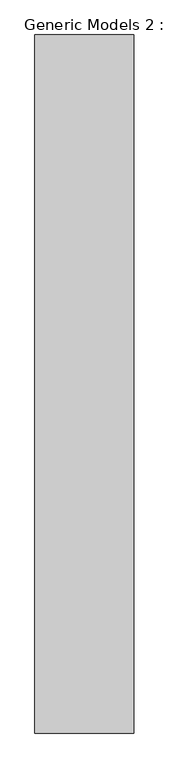
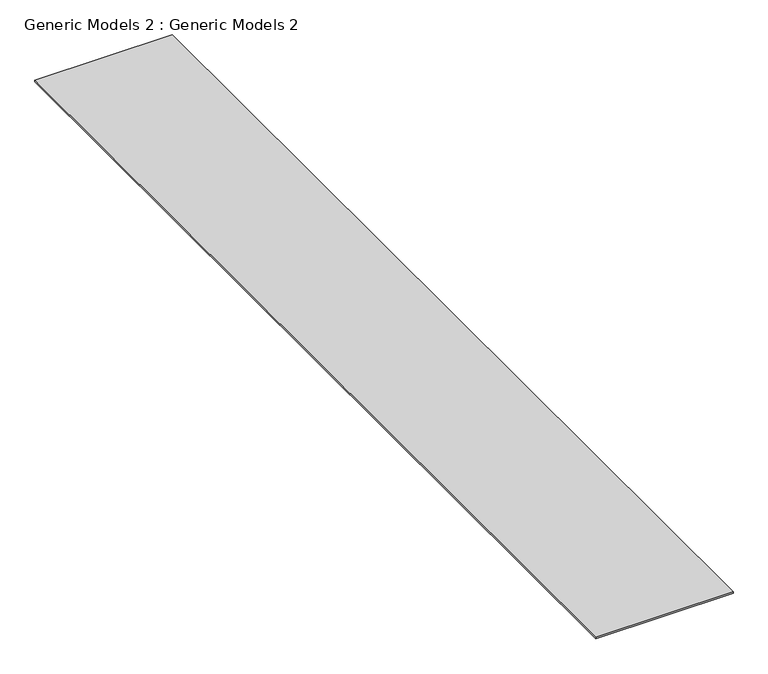
"""IFC4 building model written with IfcOpenShell, lengths in millimetres: proxy geometry, Generic Models 2 : Generic Models 2."""

from ifc_helpers import new_model, si_unit, frame, origin, place, context, project, spatial, polyline, outline, extrude, source, transform, mapped, element, save


def generic_models_2_generic_models_2_33b85b70(model_context):
    return source(origin(), model_context, "Body", "SweptSolid", [
        extrude(outline(polyline([(17947.2014317, 13822.3935985), (17947.2014317, -18476.1844555), (13375.2014317, -18476.1844555), (13375.2014317, 13822.3935985), (17947.2014317, 13822.3935985)])), frame((0.0, 0.0, -609.6), z_axis=(0.0, 0.0, 1.0), x_axis=(1.0, 0.0, 0.0)), (0.0, 0.0, 1.0), 50.8),
    ])


if __name__ == "__main__":
    model = new_model("IFC4")
    model_context = context("Model", 3, world=origin())
    ifc_project = project(units=[si_unit("LENGTHUNIT", "METRE", prefix="MILLI")], contexts=[model_context])
    site = spatial("IfcSite", under=ifc_project)
    building = spatial("IfcBuilding", under=site)
    placement = place(None, origin())
    generic_models_2_generic_models_2_shape = generic_models_2_generic_models_2_33b85b70(model_context)
    element("IfcBuildingElementProxy", 1, Name="Generic Models 2 : Generic Models 2", ObjectType="Generic Models 2 : Generic Models 2", at=placement, inside=building, context=model_context, shape_type="MappedRepresentation", body=[
        mapped(generic_models_2_generic_models_2_shape, transform((0.0, 0.0, 0.0), x_axis=(1.0, 0.0, 0.0), y_axis=(0.0, 1.0, 0.0), z_axis=(0.0, 0.0, 1.0))),
    ])
    save(model, "model.ifc")

# Revit data of these elements
# Element 1 (IfcBuildingElementProxy, "Generic Models 2 : Generic Models 2")
#   Materials on its faces: "SLAB"
# Materials
#   "SLAB": class "Generic", colour RGB 120 120 120, transparency 0, Cost = 0
